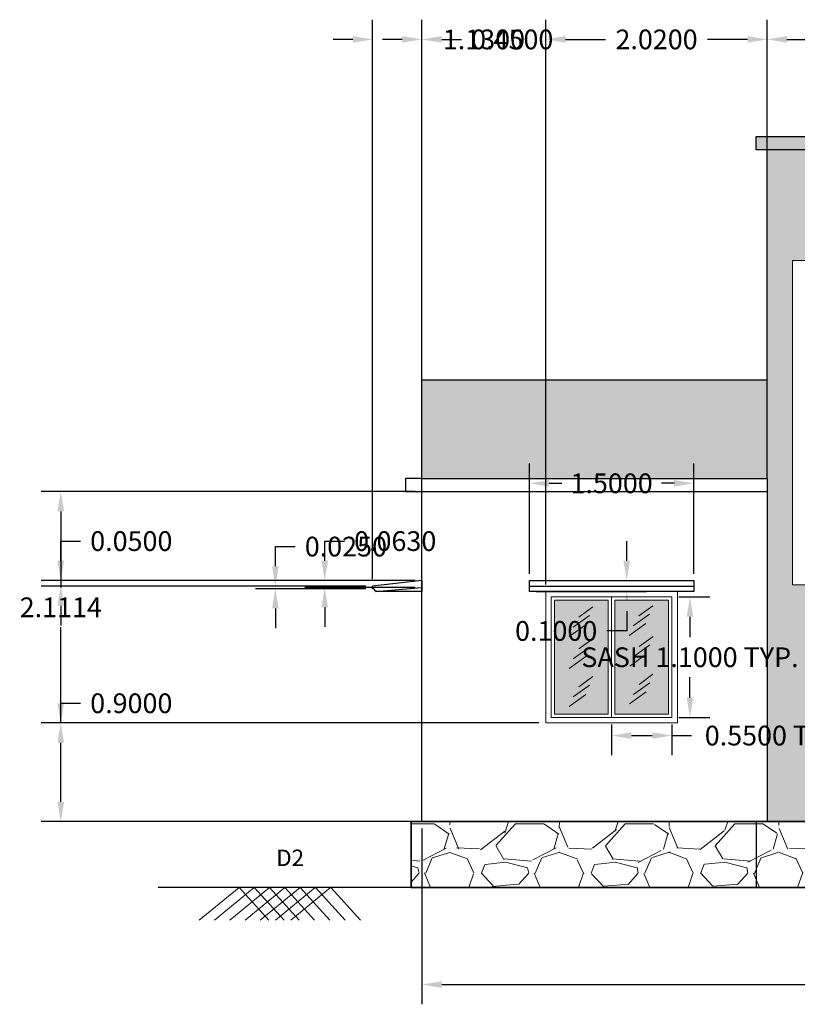
# Model space of a CAD drawing. Units: metres. Extents: x 5.2 to 41.7, y 12.2 to 37.4.
# Tile 2 of 6: x 5.2 to 12.3, y 28.4 to 37.4. Entities that reach past the tile are written whole.
import ezdxf

# ---------------------------------------------------------------- set-up
doc = ezdxf.new("R2010")
doc.units = ezdxf.units.M
doc.header["$MEASUREMENT"] = 0
for name, color, linetype, lineweight in [('A-ANNO-DIMS', 2, 'Continuous', 18), ('A-ANNO-TEXT', 3, 'Continuous', 18), ('A-ELEV', 7, 'Continuous', 25), ('A-ELEV-PATT', 9, 'Continuous', 13), ('A-FLOR-PLIN', 7, 'Continuous', 25), ('A-GLAZ-PATT', 151, 'Continuous', 13), ('A-ROOF', 7, 'Continuous', 25), ('C-TOPO', 7, 'Continuous', 25), ('C-TOPO-PATT', 8, 'Continuous', 13)]:
    doc.layers.add(name, color=color, linetype=linetype, lineweight=lineweight)
doc.layers.add('A-GLAZ', color=51, linetype='Continuous', lineweight=18, true_color=0xf7f281)
doc.layers.add('A-PLIN-PATT', color=251, linetype='Continuous', lineweight=13, true_color=0x636466)
doc.styles.get("Standard").update_dxf_attribs({"font": 'arial.ttf'})
doc.dimstyles.get("Standard").update_dxf_attribs({"dimtxt": 0.18, "dimasz": 0.18, "dimexe": 0.18, "dimexo": 0.0625, "dimgap": 0.09, "dimtad": 0, "dimtih": 1, "dimtoh": 1, "dimdec": 4, "dimzin": 0, "dimdsep": 46, "dimtxsty": 'Standard', "dimcen": 0.09, "dimadec": 0, "dimazin": 0, "dimtfac": 1, "dimtdec": 4, "dimtofl": 0, "dimtmove": 0, "dimatfit": 3, "dimfxl": 1, "dimtolj": 1, "dimtzin": 0, "dimarcsym": 0})

# ---------------------------------------------------------------- blocks, each defined once
blk = doc.blocks.new('GLASS-REFLECTION')
for p, q in [((0.08809580488861, 0.178305383476971), (0.2148507561325843, 0.2711338394228626)), ((0.0369433649416564, 0.0871027572389061), (0.184953556568928, 0.1937230376420551)), ((0.000485723746344, -2.27863267348e-05), (0.1515279092010928, 0.1087816141597138))]:
    blk.add_line(p, q)
blk = doc.blocks.new('SASH-ELEV-NARROW')
for points in [[(-0.0004402787265363, 1.099717152800995), (0.5495597212734645, 1.099717152800995), (0.5495597212734645, -0.0002828471990135), (-0.0004402787265363, -0.0002828471990135)], [(0.0295597212734649, 1.069717152800993), (0.5195597212734633, 1.069717152800993), (0.5195597212734633, 0.0297171528009876), (0.0295597212734649, 0.0297171528009876)]]:
    blk.add_lwpolyline(points, close=True)
blk = doc.blocks.new('*D22')
at = {"layer": 'A-ANNO-DIMS', "color": 0, "lineweight": -2, "transparency": 16777216}
for p, q in [((11.18205972127347, 32.09471715280101), (11.46455972127347, 32.09471715280101)), ((11.28455972127347, 31.91471715280102), (11.28455972127347, 31.7277867298815)), ((11.28455972127347, 31.174717152801), (11.28455972127347, 31.36164757572052)), ((11.18205972127347, 30.994717152801), (11.46455972127347, 30.994717152801))]:
    blk.add_line(p, q, dxfattribs=at)
at = {"layer": 'A-ANNO-DIMS', "color": 0, "lineweight": 25, "transparency": 16777216}
for points in [[(11.25455972127347, 31.91471715280102), (11.31455972127347, 31.91471715280102), (11.28455972127347, 32.09471715280101)], [(11.25455972127347, 31.174717152801), (11.31455972127347, 31.174717152801), (11.28455972127347, 30.994717152801)]]:
    blk.add_solid(points, dxfattribs=at)
at = {"layer": 'Defpoints', "color": 0, "lineweight": 25, "transparency": 16777216}
for p in [(11.11955972127347, 32.09471715280101), (11.28455972127347, 32.09471715280101), (11.11955972127347, 30.994717152801)]:
    blk.add_point(p, dxfattribs=at)
at = {"layer": 'A-ANNO-DIMS', "color": 0, "transparency": 16777216, "insert": (11.28455972127348, 31.544717152801), "char_height": 0.18, "attachment_point": 5}
blk.add_mtext('\\A1;SASH 1.1000 TYP.', dxfattribs=at)
blk = doc.blocks.new('*D23')
at = {"layer": 'A-ANNO-DIMS', "color": 0, "lineweight": -2, "transparency": 16777216}
for p, q in [((10.56955972127346, 30.93221715280099), (10.56955972127346, 30.64971715280099)), ((11.11955972127346, 30.93221715280099), (11.11955972127346, 30.64971715280099)), ((10.74955972127346, 30.82971715280099), (10.93955972127346, 30.82971715280099)), ((11.11955972127346, 30.82971715280099), (11.29955972127346, 30.82971715280099))]:
    blk.add_line(p, q, dxfattribs=at)
at = {"layer": 'A-ANNO-DIMS', "color": 0, "lineweight": 25, "transparency": 16777216}
for points in [[(10.74955972127346, 30.85971715280099), (10.74955972127346, 30.79971715280099), (10.56955972127346, 30.82971715280099)], [(10.93955972127346, 30.85971715280099), (10.93955972127346, 30.79971715280099), (11.11955972127346, 30.82971715280099)]]:
    blk.add_solid(points, dxfattribs=at)
at = {"layer": 'Defpoints', "color": 0, "lineweight": 25, "transparency": 16777216}
for p in [(10.56955972127346, 30.99471715280099), (11.11955972127346, 30.99471715280099), (11.11955972127346, 30.82971715280099)]:
    blk.add_point(p, dxfattribs=at)
at = {"layer": 'A-ANNO-DIMS', "color": 0, "transparency": 16777216, "insert": (12.07235644705791, 30.82971715280099), "char_height": 0.18, "attachment_point": 5}
blk.add_mtext('\\A1;0.5500 TYP.', dxfattribs=at)
blk = doc.blocks.new('*D37')
at = {"layer": 'A-ANNO-DIMS', "color": 0, "lineweight": -2, "transparency": 16777216}
for p, q in [((8.83956, 29.982217), (8.83956, 28.377217)), ((18.94956, 29.982217), (18.94956, 28.377217)), ((9.01956, 28.557217), (13.36978510231924, 28.557217)), ((18.76956, 28.557217), (14.41933489768076, 28.557217))]:
    blk.add_line(p, q, dxfattribs=at)
at = {"layer": 'A-ANNO-DIMS', "color": 0, "lineweight": 25, "transparency": 16777216}
for points in [[(9.01956, 28.587217), (9.01956, 28.527217), (8.83956, 28.557217)], [(18.76956, 28.587217), (18.76956, 28.527217), (18.94956, 28.557217)]]:
    blk.add_solid(points, dxfattribs=at)
at = {"layer": 'Defpoints', "color": 0, "lineweight": 25, "transparency": 16777216}
for p in [(8.83956, 30.044717), (18.94956, 30.044717), (18.94956, 28.557217)]:
    blk.add_point(p, dxfattribs=at)
at = {"layer": 'A-ANNO-DIMS', "color": 0, "transparency": 16777216, "insert": (13.89456, 28.557217), "char_height": 0.18, "attachment_point": 5}
blk.add_mtext('\\A1;10.1100', dxfattribs=at)
blk = doc.blocks.new('*D39')
at = {"layer": 'A-ANNO-DIMS', "color": 0, "lineweight": -2, "transparency": 16777216}
for p, q in [((8.83956, 32.307217), (8.83956, 37.363575)), ((9.96956, 32.207217), (9.96956, 37.363575)), ((8.65956, 37.183575), (8.479560000000001, 37.183575)), ((10.14956, 37.183575), (10.32956, 37.183575))]:
    blk.add_line(p, q, dxfattribs=at)
at = {"layer": 'A-ANNO-DIMS', "color": 0, "lineweight": 25, "transparency": 16777216}
for points in [[(8.65956, 37.213575), (8.65956, 37.153575), (8.83956, 37.183575)], [(10.14956, 37.213575), (10.14956, 37.153575), (9.96956, 37.183575)]]:
    blk.add_solid(points, dxfattribs=at)
at = {"layer": 'Defpoints', "color": 0, "lineweight": 25, "transparency": 16777216}
for p in [(9.96956, 37.183575), (8.83956, 32.244717), (9.96956, 32.144717)]:
    blk.add_point(p, dxfattribs=at)
at = {"layer": 'A-ANNO-DIMS', "color": 0, "transparency": 16777216, "insert": (9.40456, 37.183575), "char_height": 0.18, "attachment_point": 5}
blk.add_mtext('\\A1;1.1300', dxfattribs=at)
blk = doc.blocks.new('*D40')
at = {"layer": 'A-ANNO-DIMS', "color": 0, "lineweight": -2, "transparency": 16777216}
for p, q in [((9.96956, 32.207217), (9.96956, 37.363575)), ((11.98956, 34.13857500000001), (11.98956, 37.363575)), ((10.14956, 37.183575), (10.51470324693042, 37.183575)), ((11.80956, 37.183575), (11.44441675306957, 37.183575))]:
    blk.add_line(p, q, dxfattribs=at)
at = {"layer": 'A-ANNO-DIMS', "color": 0, "lineweight": 25, "transparency": 16777216}
for points in [[(10.14956, 37.213575), (10.14956, 37.153575), (9.96956, 37.183575)], [(11.80956, 37.213575), (11.80956, 37.153575), (11.98956, 37.183575)]]:
    blk.add_solid(points, dxfattribs=at)
at = {"layer": 'Defpoints', "color": 0, "lineweight": 25, "transparency": 16777216}
for p in [(11.98956, 37.183575), (11.98956, 34.07607500000001), (9.96956, 32.144717)]:
    blk.add_point(p, dxfattribs=at)
at = {"layer": 'A-ANNO-DIMS', "color": 0, "transparency": 16777216, "insert": (10.97956, 37.183575), "char_height": 0.18, "attachment_point": 5}
blk.add_mtext('\\A1;2.0200', dxfattribs=at)
blk = doc.blocks.new('*D41')
at = {"layer": 'A-ANNO-DIMS', "color": 0, "lineweight": -2, "transparency": 16777216}
for p, q in [((11.98956, 36.238575), (11.98956, 37.363575)), ((14.79956, 36.238575), (14.79956, 37.363575)), ((12.16956, 37.183575), (12.92970324693042, 37.183575)), ((14.61956, 37.183575), (13.85941675306957, 37.183575))]:
    blk.add_line(p, q, dxfattribs=at)
at = {"layer": 'A-ANNO-DIMS', "color": 0, "lineweight": 25, "transparency": 16777216}
for points in [[(12.16956, 37.213575), (12.16956, 37.153575), (11.98956, 37.183575)], [(14.61956, 37.213575), (14.61956, 37.153575), (14.79956, 37.183575)]]:
    blk.add_solid(points, dxfattribs=at)
at = {"layer": 'Defpoints', "color": 0, "lineweight": 25, "transparency": 16777216}
for p in [(14.79956, 37.183575), (11.98956, 36.176075), (14.79956, 36.176075)]:
    blk.add_point(p, dxfattribs=at)
at = {"layer": 'A-ANNO-DIMS', "color": 0, "transparency": 16777216, "insert": (13.39456, 37.183575), "char_height": 0.18, "attachment_point": 5}
blk.add_mtext('\\A1;2.8100', dxfattribs=at)
blk = doc.blocks.new('*D42')
at = {"layer": 'A-ANNO-DIMS', "color": 0, "lineweight": -2, "transparency": 16777216}
for p, q in [((8.777060000000004, 33.05607500000002), (5.364519000000004, 33.05607500000002)), ((5.544519000000003, 32.87607500000002), (5.544519000000003, 32.18076434924968)), ((5.544519000000003, 31.12471700000001), (5.544519000000003, 31.82002765075036)), ((9.907060000000003, 30.94471700000001), (5.364519000000004, 30.94471700000001))]:
    blk.add_line(p, q, dxfattribs=at)
at = {"layer": 'A-ANNO-DIMS', "color": 0, "lineweight": 25, "transparency": 16777216}
for points in [[(5.514519000000003, 32.87607500000002), (5.574519000000003, 32.87607500000002), (5.544519000000003, 33.05607500000002)], [(5.514519000000003, 31.12471700000001), (5.574519000000003, 31.12471700000001), (5.544519000000003, 30.94471700000001)]]:
    blk.add_solid(points, dxfattribs=at)
at = {"layer": 'Defpoints', "color": 0, "lineweight": 25, "transparency": 16777216}
for p in [(5.544519000000003, 33.05607500000002), (8.839560000000004, 33.05607500000002), (9.969560000000003, 30.94471700000001)]:
    blk.add_point(p, dxfattribs=at)
at = {"layer": 'A-ANNO-DIMS', "color": 0, "transparency": 16777216, "insert": (5.544519000000011, 32.00039600000001), "char_height": 0.18, "attachment_point": 5}
blk.add_mtext('\\A1;2.1114', dxfattribs=at)
blk = doc.blocks.new('*D43')
at = {"layer": 'A-ANNO-DIMS', "color": 0, "lineweight": -2, "transparency": 16777216}
for p, q in [((5.544519000000003, 30.94471700000001), (5.544519000000003, 31.12471700000001)), ((5.544519000000003, 31.12471700000001), (5.724519000000003, 31.12471700000001)), ((9.907060000000003, 30.94471700000001), (5.364519000000004, 30.94471700000001)), ((5.544519000000003, 30.22471700000001), (5.544519000000003, 30.76471700000001)), ((8.777060000000004, 30.04471700000002), (5.364519000000004, 30.04471700000001))]:
    blk.add_line(p, q, dxfattribs=at)
at = {"layer": 'A-ANNO-DIMS', "color": 0, "lineweight": 25, "transparency": 16777216}
for points in [[(5.514519000000003, 30.76471700000001), (5.574519000000003, 30.76471700000001), (5.544519000000003, 30.94471700000001)], [(5.514519000000003, 30.22471700000001), (5.574519000000003, 30.22471700000001), (5.544519000000003, 30.04471700000001)]]:
    blk.add_solid(points, dxfattribs=at)
at = {"layer": 'Defpoints', "color": 0, "lineweight": 25, "transparency": 16777216}
for p in [(5.544519000000003, 30.94471700000001), (9.969560000000003, 30.94471700000001), (8.839560000000004, 30.04471700000002)]:
    blk.add_point(p, dxfattribs=at)
at = {"layer": 'A-ANNO-DIMS', "color": 0, "transparency": 16777216, "insert": (6.187840964529343, 31.124717), "char_height": 0.18, "attachment_point": 5}
blk.add_mtext('\\A1;0.9000', dxfattribs=at)
blk = doc.blocks.new('*D70')
at = {"layer": 'A-ANNO-DIMS', "color": 0, "lineweight": -2, "transparency": 16777216}
for p, q in [((9.81956, 32.307217), (9.81956, 33.312217)), ((11.31956, 32.307217), (11.31956, 33.312217)), ((9.999559999999997, 33.132217), (10.11471006821282, 33.132217)), ((11.13956, 33.132217), (11.02440993178717, 33.132217))]:
    blk.add_line(p, q, dxfattribs=at)
at = {"layer": 'A-ANNO-DIMS', "color": 0, "lineweight": 25, "transparency": 16777216}
for points in [[(9.999559999999997, 33.162217), (9.999559999999997, 33.102217), (9.81956, 33.132217)], [(11.13956, 33.162217), (11.13956, 33.102217), (11.31956, 33.132217)]]:
    blk.add_solid(points, dxfattribs=at)
at = {"layer": 'Defpoints', "color": 0, "lineweight": 25, "transparency": 16777216}
for p in [(11.31956, 33.132217), (9.81956, 32.244717), (11.31956, 32.244717)]:
    blk.add_point(p, dxfattribs=at)
at = {"layer": 'A-ANNO-DIMS', "color": 0, "transparency": 16777216, "insert": (10.56956, 33.132217), "char_height": 0.18, "attachment_point": 5}
blk.add_mtext('\\A1;1.5000', dxfattribs=at)
blk = doc.blocks.new('*D71')
at = {"layer": 'A-ANNO-DIMS', "color": 0, "lineweight": -2, "transparency": 16777216}
for p, q in [((10.70706000000001, 32.42471700000002), (10.70706000000001, 32.60471700000002)), ((9.882060000000003, 32.24471700000002), (10.88706000000001, 32.24471700000002)), ((9.882060000000003, 32.14471700000002), (10.88706000000001, 32.14471700000002)), ((10.70706000000001, 31.96471700000002), (10.70706000000001, 31.78471700000002)), ((10.70706000000001, 31.78471700000002), (10.52706000000001, 31.78471700000002))]:
    blk.add_line(p, q, dxfattribs=at)
at = {"layer": 'A-ANNO-DIMS', "color": 0, "lineweight": 25, "transparency": 16777216}
for points in [[(10.67706000000001, 32.42471700000002), (10.73706, 32.42471700000002), (10.70706000000001, 32.24471700000002)], [(10.67706000000001, 31.96471700000002), (10.73706, 31.96471700000002), (10.70706000000001, 32.14471700000002)]]:
    blk.add_solid(points, dxfattribs=at)
at = {"layer": 'Defpoints', "color": 0, "lineweight": 25, "transparency": 16777216}
for p in [(9.819560000000003, 32.24471700000002), (9.819560000000003, 32.14471700000002), (10.70706000000001, 32.14471700000002)]:
    blk.add_point(p, dxfattribs=at)
at = {"layer": 'A-ANNO-DIMS', "color": 0, "transparency": 16777216, "insert": (10.06373803547068, 31.78471700000001), "char_height": 0.18, "attachment_point": 5}
blk.add_mtext('\\A1;0.1000', dxfattribs=at)
blk = doc.blocks.new('*D72')
at = {"layer": 'A-ANNO-DIMS', "color": 0, "lineweight": -2, "transparency": 16777216}
for p, q in [((8.38956, 32.257217), (8.38956, 37.363575)), ((8.83956, 32.307217), (8.83956, 37.363575)), ((8.20956, 37.183575), (8.02956, 37.183575)), ((9.01956, 37.183575), (9.199559999999998, 37.183575))]:
    blk.add_line(p, q, dxfattribs=at)
at = {"layer": 'A-ANNO-DIMS', "color": 0, "lineweight": 25, "transparency": 16777216}
for points in [[(8.20956, 37.213575), (8.20956, 37.153575), (8.38956, 37.183575)], [(9.01956, 37.213575), (9.01956, 37.153575), (8.83956, 37.183575)]]:
    blk.add_solid(points, dxfattribs=at)
at = {"layer": 'Defpoints', "color": 0, "lineweight": 25, "transparency": 16777216}
for p in [(8.83956, 37.183575), (8.38956, 32.194717), (8.83956, 32.244717)]:
    blk.add_point(p, dxfattribs=at)
at = {"layer": 'A-ANNO-DIMS', "color": 0, "transparency": 16777216, "insert": (9.662881964529332, 37.183575), "char_height": 0.18, "attachment_point": 5}
blk.add_mtext('\\A1;0.4500', dxfattribs=at)
blk = doc.blocks.new('*D73')
at = {"layer": 'A-ANNO-DIMS', "color": 0, "lineweight": -2, "transparency": 16777216}
for p, q in [((5.544519000000003, 32.42471700000002), (5.544519000000003, 32.60471700000002)), ((5.544519000000003, 32.60471700000002), (5.724519000000003, 32.60471700000002)), ((8.777060000000004, 32.24471700000002), (5.364519000000004, 32.24471700000002)), ((8.327060000000003, 32.19471700000001), (5.364519000000004, 32.19471700000001)), ((5.544519000000003, 32.01471700000001), (5.544519000000003, 31.83471700000001))]:
    blk.add_line(p, q, dxfattribs=at)
at = {"layer": 'A-ANNO-DIMS', "color": 0, "lineweight": 25, "transparency": 16777216}
for points in [[(5.514519000000003, 32.42471700000002), (5.574519000000003, 32.42471700000002), (5.544519000000003, 32.24471700000002)], [(5.514519000000003, 32.01471700000001), (5.574519000000003, 32.01471700000001), (5.544519000000003, 32.19471700000001)]]:
    blk.add_solid(points, dxfattribs=at)
at = {"layer": 'Defpoints', "color": 0, "lineweight": 25, "transparency": 16777216}
for p in [(5.544519000000003, 32.24471700000002), (8.389560000000003, 32.19471700000001), (8.839560000000004, 32.24471700000002)]:
    blk.add_point(p, dxfattribs=at)
at = {"layer": 'A-ANNO-DIMS', "color": 0, "transparency": 16777216, "insert": (6.187840964529343, 32.60471700000001), "char_height": 0.18, "attachment_point": 5}
blk.add_mtext('\\A1;0.0500', dxfattribs=at)
blk = doc.blocks.new('*D74')
at = {"layer": 'A-ANNO-DIMS', "color": 0, "lineweight": -2, "transparency": 16777216}
for p, q in [((7.952060000000007, 32.42471700000002), (7.952060000000007, 32.60471700000002)), ((7.952060000000007, 32.60471700000002), (8.132060000000008, 32.60471700000002)), ((8.777060000000004, 32.24471700000002), (7.772060000000007, 32.24471700000002)), ((8.777060000000004, 32.18171800000001), (7.772060000000007, 32.18171800000001)), ((7.952060000000007, 32.00171800000001), (7.952060000000007, 31.82171800000001))]:
    blk.add_line(p, q, dxfattribs=at)
at = {"layer": 'A-ANNO-DIMS', "color": 0, "lineweight": 25, "transparency": 16777216}
for points in [[(7.922060000000007, 32.42471700000002), (7.982060000000007, 32.42471700000002), (7.952060000000007, 32.24471700000002)], [(7.922060000000007, 32.00171800000001), (7.982060000000007, 32.00171800000001), (7.952060000000007, 32.18171800000001)]]:
    blk.add_solid(points, dxfattribs=at)
at = {"layer": 'Defpoints', "color": 0, "lineweight": 25, "transparency": 16777216}
for p in [(7.952060000000007, 32.24471700000002), (8.839560000000004, 32.24471700000002), (8.839560000000004, 32.18171800000001)]:
    blk.add_point(p, dxfattribs=at)
at = {"layer": 'A-ANNO-DIMS', "color": 0, "transparency": 16777216, "insert": (8.595381964529347, 32.60471700000001), "char_height": 0.18, "attachment_point": 5}
blk.add_mtext('\\A1;0.0630', dxfattribs=at)
blk = doc.blocks.new('*D75')
at = {"layer": 'A-ANNO-DIMS', "color": 0, "lineweight": -2, "transparency": 16777216}
for p, q in [((7.502060000000007, 32.37471700000001), (7.502060000000007, 32.55471700000001)), ((7.502060000000007, 32.55471700000001), (7.682060000000006, 32.55471700000001)), ((8.327060000000003, 32.19471700000001), (7.322060000000007, 32.19471700000001)), ((8.327060000000003, 32.16971700000001), (7.322060000000007, 32.16971700000001)), ((7.502060000000007, 31.98971700000001), (7.502060000000007, 31.80971700000001))]:
    blk.add_line(p, q, dxfattribs=at)
at = {"layer": 'A-ANNO-DIMS', "color": 0, "lineweight": 25, "transparency": 16777216}
for points in [[(7.472060000000007, 32.37471700000001), (7.532060000000007, 32.37471700000001), (7.502060000000007, 32.19471700000001)], [(7.472060000000007, 31.98971700000001), (7.532060000000007, 31.98971700000001), (7.502060000000007, 32.16971700000001)]]:
    blk.add_solid(points, dxfattribs=at)
at = {"layer": 'Defpoints', "color": 0, "lineweight": 25, "transparency": 16777216}
for p in [(7.502060000000007, 32.19471700000001), (8.389560000000003, 32.19471700000001), (8.389560000000003, 32.16971700000001)]:
    blk.add_point(p, dxfattribs=at)
at = {"layer": 'A-ANNO-DIMS', "color": 0, "transparency": 16777216, "insert": (8.145381964529346, 32.55471700000001), "char_height": 0.18, "attachment_point": 5}
blk.add_mtext('\\A1;0.0250', dxfattribs=at)

msp = doc.modelspace()

# ---------------------------------------------------------------- hatches: boundary and pattern name
at = {"layer": 'A-ELEV-PATT'}
h = msp.add_hatch(color=256, dxfattribs=at)
h.dxf.hatch_style = 1
h.paths.add_polyline_path([(14.89955972127346, 36.29607479937437), (11.88955972127345, 36.29607479937437), (11.88955972127345, 36.17607479937438), (14.89955972127346, 36.17607479937438)])
h.paths.add_polyline_path([(11.98955972127346, 34.07607479937438), (8.839559721273464, 34.07607479937438), (8.839559721273464, 33.17607479937438), (11.98955972127346, 33.17607479937438)])
h.paths.add_polyline_path([(18.94955972127346, 34.07607479937438), (14.79955972127346, 34.07607479937438), (14.79955972127346, 33.17607479937438), (18.94955972127346, 33.17607479937438)])
h = msp.add_hatch(color=256, dxfattribs=at)
h.dxf.hatch_style = 1
h.paths.add_polyline_path([(14.79955972127346, 32.144717152801), (14.79955972127346, 33.17607479937438), (14.79955972127346, 36.17607479937438), (11.98955972127346, 36.17607479937438), (11.98955972127346, 33.17607479937438), (11.98955972127346, 30.04471715280099), (14.79955972127346, 30.044717152801)])
h.paths.add_polyline_path([(12.21955972127346, 32.204717152801), (12.21955972127346, 35.164717152801), (14.56955972127346, 35.164717152801), (14.56955972127346, 32.204717152801)], flags=16)
h.paths.add_polyline_path([(12.26955972127346, 32.254717152801), (12.26955972127346, 33.684717152801), (12.26955972127346, 35.114717152801), (13.39455972127346, 35.114717152801), (14.51955972127345, 35.114717152801), (14.51955972127345, 33.684717152801), (14.51955972127345, 32.254717152801), (13.39455972127346, 32.254717152801)], flags=0)
h.paths.add_polyline_path([(12.26955972127346, 32.25471715280099), (12.26955972127346, 35.114717152801), (14.51955972127346, 35.114717152801), (14.51955972127346, 32.25471715280099)], flags=0)
h.paths.add_polyline_path([(12.31955972127346, 32.304717152801), (12.31955972127346, 33.63471715280101), (13.34455972127346, 33.63471715280101), (13.34455972127346, 32.304717152801)], flags=0)
h.paths.add_polyline_path([(13.44455972127346, 32.304717152801), (13.44455972127346, 33.63471715280101), (14.46955972127345, 33.63471715280101), (14.46955972127345, 32.304717152801)], flags=0)
h.paths.add_polyline_path([(12.31955972127346, 33.734717152801), (12.31955972127346, 35.064717152801), (13.34455972127346, 35.064717152801), (13.34455972127346, 33.734717152801)], flags=0)
h.paths.add_polyline_path([(13.44455972127346, 33.734717152801), (13.44455972127346, 35.064717152801), (14.46955972127345, 35.064717152801), (14.46955972127345, 33.734717152801)], flags=0)
h = msp.add_hatch(color=256, dxfattribs=at)
h.dxf.hatch_style = 1
h.paths.add_polyline_path([(14.79955972127346, 32.144717152801), (14.79955972127346, 33.17607479937438), (14.79955972127346, 36.17607479937438), (11.98955972127346, 36.17607479937438), (11.98955972127346, 33.17607479937438), (11.98955972127346, 30.04471715280099), (14.79955972127346, 30.044717152801)])
h.paths.add_polyline_path([(12.21955972127346, 32.204717152801), (12.21955972127346, 35.164717152801), (14.56955972127346, 35.164717152801), (14.56955972127346, 32.204717152801)], flags=16)
h.paths.add_polyline_path([(13.39455972127346, 32.254717152801), (12.26955972127346, 32.254717152801), (12.26955972127346, 33.684717152801), (12.26955972127346, 35.114717152801), (13.39455972127346, 35.114717152801), (14.51955972127345, 35.114717152801), (14.51955972127345, 33.684717152801), (14.51955972127345, 32.254717152801)], flags=0)
h.paths.add_polyline_path([(12.26955972127346, 32.25471715280099), (12.26955972127346, 35.114717152801), (14.51955972127346, 35.114717152801), (14.51955972127346, 32.25471715280099)], flags=0)
h.paths.add_polyline_path([(13.44455972127346, 32.304717152801), (13.44455972127346, 33.63471715280101), (14.46955972127345, 33.63471715280101), (14.46955972127345, 32.304717152801)], flags=0)
h.paths.add_polyline_path([(13.34455972127346, 32.304717152801), (12.31955972127346, 32.304717152801), (12.31955972127346, 33.63471715280101), (13.34455972127346, 33.63471715280101)], flags=0)
h.paths.add_polyline_path([(13.44455972127346, 33.734717152801), (13.44455972127346, 35.064717152801), (14.46955972127345, 35.064717152801), (14.46955972127345, 33.734717152801)], flags=0)
h.paths.add_polyline_path([(13.34455972127346, 33.734717152801), (12.31955972127346, 33.734717152801), (12.31955972127346, 35.064717152801), (13.34455972127346, 35.064717152801)], flags=0)
at = {"layer": 'A-GLAZ-PATT'}
h = msp.add_hatch(color=256, dxfattribs=at)
h.dxf.hatch_style = 1
h.set_gradient(color1=(173, 221, 247), color2=(199, 200, 202))
h.paths.add_polyline_path([(10.53955972127346, 32.064717152801), (10.04955972127346, 32.064717152801), (10.04955972127346, 31.02471715280099), (10.53955972127346, 31.02471715280099)])
h.paths.add_polyline_path([(11.08955972127346, 32.064717152801), (10.59955972127346, 32.064717152801), (10.59955972127346, 31.02471715280099), (11.08955972127346, 31.02471715280099)])
at = {"layer": 'A-PLIN-PATT'}
h = msp.add_hatch(dxfattribs=at)
h.set_pattern_fill('GRAVEL', color=256)
h.set_pattern_definition([(228.012787504, (-11.19360896471565, -4.432464084464029), (-8.000000000000062, -9.000000000000004), [0.134536, -13.3190880470737]), (184.969740728, (-11.28360896471565, -4.532464084464029), (11.99999999999997, 1.000000000000035), [0.230868, -22.85592476122999]), (132.510447078, (-11.51360896471565, -4.55246408446403), (10.00000000000011, -10.99999999999986), [0.162788, -16.1160325960997]), (267.273689006, (-11.90360896471565, -4.80246408446403), (1.000000000000024, 20.00000000000002), [0.210238, -20.813558041629]), (292.833654178, (-11.91360896471565, -5.01246408446403), (-4.999999999999988, 12.00000000000003), [0.2061549999999999, -20.40937312808829]), (357.273689006, (-11.83360896471565, -5.202464084464029), (-20.00000000000002, 1.000000000000025), [0.210238, -20.813558041629]), (37.6942404667, (-11.62360896471565, -5.21246408446403), (-13, -9.999999999999973), [0.278029, -27.524848548916]), (72.2553283749, (-11.40360896471565, -5.04246408446403), (7.000000000000027, 22.00000000000001), [0.2624879999999999, -25.98632149681339]), (121.429565615, (-11.32360896471565, -4.79246408446403), (-8.00000000000002, 12.99999999999999), [0.21095, -20.884073109729]), (175.236358309, (-11.43360896471565, -4.612464084464029), (10.99999999999998, -1.000000000000037), [0.240832, -11.8007625787923]), (222.397437798, (-11.67360896471565, -4.59246408446403), (-11.99999999999996, -10.99999999999997), [0.311448, -30.8333750047949]), (138.814074834, (-10.91360896471565, -4.812464084464029), (-7.000000000000032, 6), [0.106301, -10.52384481273469]), (171.46923439, (-10.99360896471565, -4.74246408446403), (13, -1.999999999999995), [0.202237, -20.021511416157]), (225, (-11.19360896471565, -4.71246408446403), (-1e-16, -0.9999999999999328), [0.141421, -1.2727925623731]), (203.198590514, (-11.26360896471565, -4.59246408446403), (4.999999999999989, 1.999999999999975), [0.076158, -7.5396151058639]), (291.801409486, (-11.33360896471565, -4.622464084464029), (-0.9999999999996839, 3.000000000000102), [0.107703, -5.2774618071345]), (30.96375653209999, (-11.29360896471565, -4.722464084464029), (3.000000000000053, 1.999999999999979), [0.174929, -5.656022894845299]), (161.565051177, (-11.14360896471565, -4.63246408446403), (2.000000000000011, -0.9999999999999767), [0.1264909999999999, -3.035786660168398]), (16.389540334, (-11.91360896471565, -4.622464084464029), (9.999999999999966, 3.000000000000043), [0.1772, -17.5428451466694]), (70.3461759419, (-11.74360896471565, -4.572464084464029), (-4.00000000000122, -11.00000000000339), [0.148661, -14.717407747319]), (293.198590514, (-11.14360896471565, -4.432464084464029), (-1.99999999999997, 4.999999999999991), [0.152315, -7.4634581058639]), (343.610459666, (-11.08360896471565, -4.572464084464029), (-9.999999999999966, 3.000000000000043), [0.1771999999999999, -17.54284514666899]), (339.44395478, (-11.91360896471565, -5.242464084464029), (-5.000000000000036, 2.000000000000024), [0.1708799999999999, -8.373123745317496]), (294.775140569, (-11.75360896471565, -5.30246408446403), (-5.000000000000005, 11), [0.143178, -14.174643063276]), (66.8014094864, (-11.13360896471565, -5.432464084464029), (1.999999999999981, 4.999999999999969), [0.152315, -7.4634581058639]), (17.3540246363, (-11.07360896471565, -5.29246408446403), (-12.99999999999998, -3.999999999999962), [0.167631, -16.59542361424]), (69.4439547804, (-11.62360896471565, -5.432464084464029), (-2.000000000000007, -4.999999999999954), [0.08544, -8.458563745317496]), (101.3099324739999, (-11.19360896471565, -5.432464084464029), (-0.9999999999999637, 4.000000000000012), [0.05099, -5.048029513592799]), (165.963756532, (-11.20360896471565, -5.38246408446403), (2.999999999999958, -1.000000000000001), [0.206155, -3.9169506256177]), (186.009005957, (-11.40360896471565, -5.33246408446403), (10.00000000000004, 0.9999999999999831), [0.19105, -18.9139231745428]), (303.690067526, (-11.29360896471565, -4.812464084464029), (-0.9999999999999872, 1.999999999999985), [0.1442219999999999, -3.461329275463999]), (353.157226587, (-11.21360896471565, -4.932464084464029), (17.00000000000001, -2.000000000000052), [0.251794, -24.9275626240283]), (60.9453959009, (-10.96360896471565, -4.96246408446403), (-3.999999999999975, -6.999999999999976), [0.102956, -10.192674140987]), (90, (-10.91360896471565, -4.872464084464029), (-0.9999999999999998, 1), [0.06, -0.9399999999999998]), (120.256437164, (-11.42360896471565, -5.30246408446403), (4.000000000000008, -7.000000000000007), [0.138924, -13.7535199894498]), (48.01278750419999, (-11.49360896471565, -5.182464084464029), (8, 8.999999999999975), [0.269072, -13.1845520470737]), (0, (-11.31360896471565, -4.982464084464029), (1, 1), [0.26, -0.7400000000000001]), (325.304846469, (-11.05360896471565, -4.982464084464029), (10.00000000000014, -6.999999999999825), [0.1581139999999999, -15.65327430084199]), (254.0546040990001, (-10.92360896471565, -5.072464084464029), (-1.000000000000037, -4.000000000000004), [0.145602, -7.1345078892805]), (207.645975364, (-10.96360896471565, -5.21246408446403), (-18.99999999999995, -10.00000000000005), [0.237065, -23.4694741822594]), (175.42607874, (-11.17360896471565, -5.322464084464029), (-12.99999999999995, 1.000000000000001), [0.250799, -24.8290734079689])])
h.paths.add_polyline_path([(11.88955972127345, 30.04471715280099), (8.739559721273462, 30.04471715280099), (8.739559721273462, 29.44471715280099), (11.88955972127345, 29.44471715280099)])
h.paths.add_polyline_path([(14.89955972127346, 30.04471715280099), (11.88955972127345, 30.04471715280099), (11.88955972127345, 29.44471715280099), (14.89955972127346, 29.44471715280099)])
h.paths.add_polyline_path([(18.54752032864311, 30.04471715280099), (15.99955972127346, 30.04471715280099), (15.99955972127346, 29.89471715280099), (16.29955972127345, 29.89471715280099), (16.29955972127345, 29.74471715280099), (16.59955972127345, 29.74471715280099), (16.59955972127345, 29.59471715280099), (16.89955972127346, 29.59471715280099), (16.89955972127346, 29.44471715280099), (18.54752032864311, 29.44471715280099)])
h.paths.add_polyline_path([(19.04955972127346, 30.04471715280099), (18.84752032864312, 30.04471715280099), (18.84752032864312, 29.44471715280099), (19.04955972127346, 29.44471715280099)])
at = {"layer": 'C-TOPO-PATT'}
h = msp.add_hatch(dxfattribs=at)
h.set_pattern_fill('ANSI31', color=256, scale=0.7098185496078938, angle=-5.360993184015256, style=0)
h.set_pattern_definition([(39.63900681598474, (0, 0), (-0.0566034514788392, 0.0683270544114787), [])])
h.paths.add_polyline_path([(6.808192, 29.144699), (7.656582, 29.144699), (8.01874, 29.444717), (7.170348999999999, 29.444717)])
h = msp.add_hatch(dxfattribs=at)
h.set_pattern_fill('ANSI31', color=256, scale=0.828315939655125, angle=87.08559131637921, style=0)
h.set_pattern_definition([(132.0855913163792, (0, 0), (-0.0768412561320785, -0.069396310091206), [])])
h.paths.add_polyline_path([(7.170348999999999, 29.444717), (7.4413, 29.144699), (8.28969, 29.144699), (8.01874, 29.444717)])

# ---------------------------------------------------------------- linework, layer by layer
at = {"layer": 'A-ELEV'}
for p, q in [((11.98955972127346, 33.17607479937438), (11.98955972127346, 36.17607479937438)), ((8.839559721273464, 33.17607479937438), (8.839559721273464, 34.07607479937438)), ((8.839559721273464, 34.07607479937438), (11.98955972127346, 34.07607479937438)), ((11.98955972127346, 33.17607479937438), (11.98955972127346, 30.04471715280099)), ((8.839559721273464, 30.04471715280099), (8.839559721273464, 33.05607479937439))]:
    msp.add_line(p, q, dxfattribs=at)
at = {"layer": 'A-FLOR-PLIN'}
for p, q in [((8.839559721273464, 30.04471715280099), (8.739559721273462, 30.04471715280099)), ((8.739559721273462, 30.04471715280099), (8.739559721273462, 29.44471715280099)), ((18.54752032864311, 30.044717152801), (8.739559721273462, 30.04471715280099)), ((11.88955972127345, 30.04471715280099), (11.88955972127345, 29.44471715280099)), ((8.739559721273462, 29.44471715280099), (19.04955972127346, 29.44471715280099))]:
    msp.add_line(p, q, dxfattribs=at)
msp.add_lwpolyline([(18.84752032864312, 30.04471715280099), (19.04955972127346, 30.04471715280099), (19.04955972127346, 29.44471715280099), (8.739559721273462, 29.44471715280099), (8.739559721273462, 30.04471715280099), (18.54752032864311, 30.04471715280099)], dxfattribs=at)
at = {"layer": 'A-GLAZ'}
for points in [[(12.21955972127346, 35.164717152801), (14.56955972127346, 35.164717152801), (14.56955972127346, 32.204717152801), (12.21955972127346, 32.204717152801)], [(9.969559721273463, 32.144717152801), (11.16955972127346, 32.144717152801), (11.16955972127346, 30.94471715280099), (9.969559721273463, 30.94471715280099)], [(10.01955972127346, 32.094717152801), (11.11955972127346, 32.094717152801), (11.11955972127346, 30.99471715280099), (10.01955972127346, 30.99471715280099)]]:
    msp.add_lwpolyline(points, close=True, dxfattribs=at)
at = {"layer": 'A-ROOF'}
for p, q in [((8.839559721273464, 33.17607479937438), (8.689559721273463, 33.17607479937438)), ((8.689559721273463, 33.17607479937438), (8.689559721273463, 33.05607479937439)), ((8.839559721273464, 33.17607479937438), (11.98955972127346, 33.17607479937438)), ((8.689559721273463, 33.05607479937439), (8.839559721273464, 33.05607479937439)), ((8.839559721273464, 33.05607479937439), (11.88955972127345, 33.05607479937438)), ((11.88955972127345, 33.05607479937438), (11.98955972127346, 33.05607479937438)), ((8.839559721273464, 32.24471715280099), (8.389559721273464, 32.19471715280099)), ((8.414559721273463, 32.144717152801), (8.839559721273464, 32.18171835099751)), ((9.819559721273462, 32.19471715280099), (11.31955972127346, 32.19471715280099))]:
    msp.add_line(p, q, dxfattribs=at)
for points in [[(11.88955972127345, 36.29607479937437), (14.89955972127346, 36.29607479937437), (14.89955972127346, 36.17607479937438), (11.88955972127345, 36.17607479937438)], [(9.819559721273462, 32.24471715280099), (11.31955972127346, 32.24471715280099), (11.31955972127346, 32.144717152801), (9.819559721273462, 32.144717152801)]]:
    msp.add_lwpolyline(points, close=True, dxfattribs=at)
for points in [[(8.389559721273464, 32.16971715280099), (8.389559721273464, 32.19471715280099)], [(8.839559721273464, 32.24471715280099), (8.839559721273464, 32.144717152801), (8.414559721273463, 32.144717152801)]]:
    msp.add_lwpolyline(points, dxfattribs=at)
msp.add_arc((8.389559721273464, 32.144717152801), 0.0249999999999986, 0, 90, dxfattribs=at)
at = {"layer": 'C-TOPO'}
msp.add_line((8.739559721273462, 29.44471715280099), (6.43201908822948, 29.44471715280099), dxfattribs=at)

# ---------------------------------------------------------------- block references
at = {"layer": 'A-GLAZ'}
for p in [(10.02, 30.995), (10.57, 30.995)]:
    msp.add_blockref('SASH-ELEV-NARROW', p, dxfattribs=at)
at = {"layer": 'A-GLAZ-PATT'}
for p in [(10.183, 31.733), (10.72931799240084, 31.74335538374309), (10.73425800299717, 31.46441474482433), (10.18334492762821, 31.44219819921379), (10.18334492762821, 31.09660792346356), (10.731787997699, 31.11882446907405)]:
    msp.add_blockref('GLASS-REFLECTION', p, dxfattribs=at)

# ---------------------------------------------------------------- texts
at = {"layer": 'A-ANNO-TEXT', "insert": (6.712809543650394, 29.78903202615662), "char_height": 0.15, "attachment_point": 1}
msp.add_mtext_dynamic_manual_height_columns('\\pxqc;{D2}', width=1.848326114625081, gutter_width=1, heights=[0], dxfattribs=at)

# ---------------------------------------------------------------- dimensions: what is measured, and where the dimension line sits
at = {"layer": 'A-ANNO-DIMS'}
for base, p1, p2, picture, middle in [((8.83956, 37.183575), (8.38956, 32.194717), (8.83956, 32.244717), '*D72', (9.662881964529332, 37.183575)), ((9.96956, 37.183575), (8.83956, 32.244717), (9.96956, 32.144717), '*D39', (9.40456, 37.183575)), ((11.98956, 37.183575), (9.96956, 32.144717), (11.98956, 34.07607500000001), '*D40', (10.97956, 37.183575)), ((14.79956, 37.183575), (11.98956, 36.176075), (14.79956, 36.176075), '*D41', (13.39456, 37.183575)), ((11.31956, 33.132217), (9.81956, 32.244717), (11.31956, 32.244717), '*D70', (10.56956, 33.132217)), ((18.94956, 28.557217), (8.83956, 30.044717), (18.94956, 30.044717), '*D37', (13.89456, 28.557217))]:
    dim = msp.add_linear_dim(base=base, p1=p1, p2=p2, dimstyle='Standard', override={"dimdec": 4, "dimlfac": 1, "dimrnd": 0, "dimzin": 0, "dimdsep": 46, "dimlunit": 2}, dxfattribs=at)
    dim.commit()
    dim.dimension.update_dxf_attribs({"geometry": picture, "text_midpoint": middle})
for base, p1, p2, angle, picture, middle in [((5.544519000000003, 33.05607500000002), (9.96956, 30.944717), (8.83956, 33.056075), 90, '*D42', (5.544519000000011, 32.00039600000001)), ((5.544519000000003, 32.24471700000002), (8.38956, 32.194717), (8.83956, 32.244717), 90, '*D73', (6.187840964529343, 32.60471700000001)), ((7.952060000000007, 32.24471700000002), (8.83956, 32.181718), (8.83956, 32.244717), 90, '*D74', (8.595381964529347, 32.60471700000001)), ((7.502060000000007, 32.19471700000001), (8.38956, 32.169717), (8.38956, 32.194717), 90, '*D75', (8.145381964529346, 32.55471700000001)), ((10.70706000000001, 32.14471700000002), (9.81956, 32.244717), (9.81956, 32.144717), 270, '*D71', (10.06373803547068, 31.78471700000001)), ((5.544519000000003, 30.94471700000001), (8.83956, 30.044717), (9.96956, 30.944717), 90, '*D43', (6.187840964529343, 31.124717))]:
    dim = msp.add_linear_dim(base=base, p1=p1, p2=p2, angle=angle, dimstyle='Standard', override={"dimdec": 4, "dimlfac": 1, "dimrnd": 0, "dimzin": 0, "dimdsep": 46, "dimlunit": 2}, dxfattribs=at)
    dim.commit()
    dim.dimension.update_dxf_attribs({"geometry": picture, "text_midpoint": middle})
dim = msp.add_linear_dim(base=(11.28455972127347, 32.09471715280101), p1=(11.11955972127346, 30.99471715280099), p2=(11.11955972127346, 32.094717152801), angle=90, text='SASH <> TYP.', dimstyle='Standard', override={"dimdec": 4, "dimlfac": 1, "dimrnd": 0, "dimzin": 0, "dimdsep": 46, "dimlunit": 2}, dxfattribs=at)
dim.commit()
dim.dimension.update_dxf_attribs({"geometry": '*D22', "text_midpoint": (11.28455972127348, 31.544717152801)})
dim = msp.add_linear_dim(base=(11.11955972127346, 30.82971715280099), p1=(10.56955972127346, 30.99471715280099), p2=(11.11955972127346, 30.99471715280099), text='<> TYP.', dimstyle='Standard', override={"dimdec": 4, "dimlfac": 1, "dimrnd": 0, "dimzin": 0, "dimdsep": 46, "dimlunit": 2}, dxfattribs=at)
dim.commit()
dim.dimension.update_dxf_attribs({"geometry": '*D23', "text_midpoint": (12.07235644705791, 30.82971715280099)})

doc.saveas('drawing.dxf')
